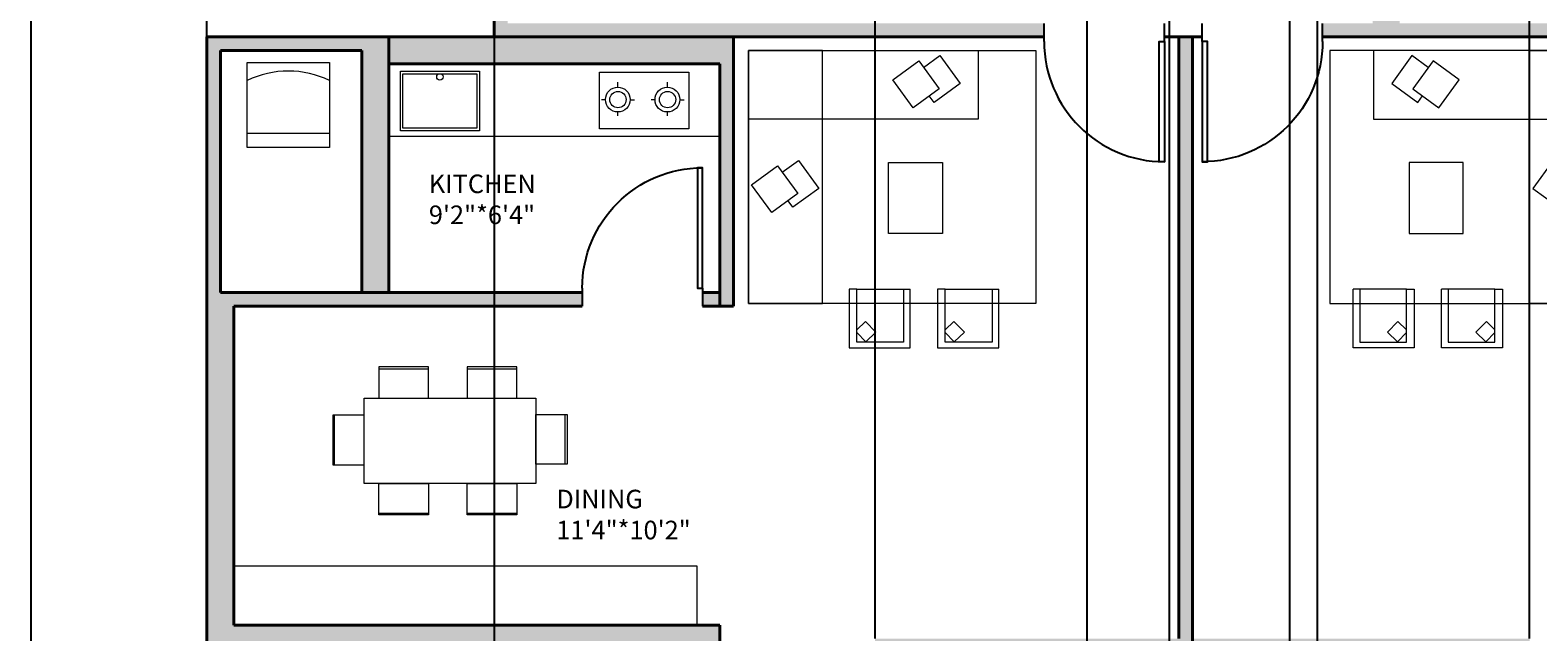
# Model space of a CAD drawing. Units: inches. Extents: x 1642 to 2399, y 1011 to 2291.
# Tile 2 of 7: x 1642 to 2143, y 1395 to 1595. Entities that reach past the tile are written whole.
import ezdxf

# ---------------------------------------------------------------- set-up
doc = ezdxf.new("R2010")
doc.units = ezdxf.units.IN
for name, color, linetype, lineweight in [('A-ANNO-DIMS', 2, 'Continuous', 18), ('A-AREA-IDEN', 7, 'Continuous', 20), ('A-DOOR', 4, 'Continuous', 25), ('A-EQPM', 8, 'Continuous', 18), ('A-FLOR-CASE', 30, 'Continuous', 18), ('A-FLOR-FIXT', 9, 'Continuous', 18), ('A-FURN', 8, 'Continuous', 18), ('A-WALL-PATT', 40, 'Continuous', 13), ('WALL', 40, 'Continuous', 40)]:
    doc.layers.add(name, color=color, linetype=linetype, lineweight=lineweight)
doc.styles.get("Standard").update_dxf_attribs({"font": 'arial.ttf'})
doc.dimstyles.get("Standard").update_dxf_attribs({"dimtxt": 0.18, "dimasz": 0.18, "dimexe": 0.18, "dimexo": 0.0625, "dimgap": 0.09, "dimtad": 0, "dimtih": 1, "dimtoh": 1, "dimdec": 4, "dimzin": 0, "dimdsep": 46, "dimtxsty": 'Standard', "dimcen": 0.09, "dimadec": 0, "dimazin": 0, "dimtfac": 1, "dimtdec": 4, "dimtofl": 0, "dimtmove": 0, "dimatfit": 3, "dimfxl": 1, "dimtolj": 1, "dimtzin": 0, "dimarcsym": 0})

# ---------------------------------------------------------------- blocks, each defined once
blk = doc.blocks.new('*U2')
for p, q in [((0, 0), (0, -6)), ((40, 0), (40, -6))]:
    blk.add_line(p, q)
blk.add_lwpolyline([(0, 0), (0, 40), (1.75, 40), (1.75, 0)], close=True)
blk.add_arc((0, 0), 40, 0, 90)
blk = doc.blocks.new('TABLE-DINING-SIX-SEAT')
for p, q in [((15.31, 48.55), (31.81, 48.55)), ((44.68, 48.55), (61.18, 48.55)), ((0.59, 16.67), (0.59, 33.17)), ((77.22, 16.83), (77.22, 33.33)), ((15.31, 0.59), (31.81, 0.59)), ((44.68, 0.59), (61.18, 0.59))]:
    blk.add_line(p, q)
for points in [[(15.31, 38.77), (31.81, 38.77), (31.81, 49.15), (15.31, 49.15)], [(44.68, 38.77), (61.18, 38.77), (61.18, 49.15), (44.68, 49.15)], [(10.38, 38.77), (67.43, 38.77), (67.43, 10.38), (10.38, 10.38)], [(10.38, 16.67), (10.38, 33.17), (0, 33.17), (0, 16.67)], [(67.43, 16.83), (67.43, 33.33), (77.81, 33.33), (77.81, 16.83)], [(15.31, 10.38), (31.81, 10.38), (31.81, 0), (15.31, 0)], [(44.68, 10.38), (61.18, 10.38), (61.18, 0), (44.68, 0)]]:
    blk.add_lwpolyline(points, close=True)
blk = doc.blocks.new('SEATING-CORNER')
for points in [[(0, 84.13), (76.26, 84.13), (76.26, 61.34), (0, 61.34)], [(0, 0), (24.56, 0), (24.56, 84.13), (0, 84.13)], [(56.51, 80.66), (63.26, 71.39), (54.61, 65.09), (47.86, 74.37)], [(9.57, 45.8), (16.32, 36.53), (7.67, 30.23), (0.92, 39.51)]]:
    blk.add_lwpolyline(points, close=True)
for points in [[(58.1, 78.48), (63.51, 82.42), (70.26, 73.15), (61.61, 66.85), (60.02, 69.03)], [(11.16, 43.62), (16.57, 47.56), (23.32, 38.28), (14.67, 31.99), (13.08, 34.17)]]:
    blk.add_lwpolyline(points)
blk = doc.blocks.new('CHAIR-LOUNGE')
for p, q in [((2.54, 19.51), (0, 19.51)), ((0, 19.51), (0, 0)), ((18.08, 19.51), (20.31, 19.51)), ((20.31, 19.32), (20.31, 19.51)), ((20.31, 0), (20.31, 19.32)), ((0, 0), (20.31, 0))]:
    blk.add_line(p, q)
blk.add_lwpolyline([(2.54, 19.51), (18.08, 19.51), (18.08, 1.93), (2.54, 1.93)], close=True)
blk.add_lwpolyline([(2.54, 6.05), (5.4, 8.82), (8.88, 5.23), (5.55, 2), (2.54, 5.1)])
blk = doc.blocks.new('COOKTOP-TWO-BURNER')
for p, q in [((6.17, 13.89), (6.17, 15.59)), ((22.64, 13.89), (22.64, 15.59)), ((2, 9.67), (0.69, 9.67)), ((6.02, 5.65), (6.02, 4.35)), ((10.24, 9.72), (11.69, 9.72)), ((18.47, 9.67), (17.17, 9.67)), ((22.49, 5.65), (22.49, 4.35)), ((26.71, 9.72), (28.17, 9.72))]:
    blk.add_line(p, q)
blk.add_lwpolyline([(0, 18.89), (29.66, 18.89), (29.66, 0), (0, 0)], close=True)
for centre, radius in [((6.12, 9.77), 4.12), ((6.17, 9.77), 2.71), ((22.59, 9.77), 4.12), ((22.64, 9.77), 2.71)]:
    blk.add_circle(centre, radius)
blk = doc.blocks.new('SINK-KITCHEN-SINGLE')
for points in [[(0, 19.82), (26.24, 19.82), (26.24, 0), (0, 0)], [(0.83, 18.98), (25.41, 18.98), (25.41, 0.83), (0.83, 0.83)]]:
    blk.add_lwpolyline(points, close=True)
blk.add_circle((13.12, 17.93), 1.05)
blk = doc.blocks.new('UTILITY-APPLIANCE')
blk.add_line((0, 4.7), (27.35, 4.7))
blk.add_lwpolyline([(0, 28.26), (27.35, 28.26), (27.35, 0), (0, 0)], close=True)
blk.add_arc((13.68, -6.28), 31.65, 64.3994, 115.6006)
blk = doc.blocks.new('TABLE-COFFEE')
blk.add_lwpolyline([(0, 23.65), (17.89, 23.65), (17.89, 0), (0, 0)], close=True)
blk = doc.blocks.new('*D33')
at = {"layer": 'A-ANNO-DIMS', "color": 0, "lineweight": -2, "transparency": 16777216}
for p, q in [((1700.65, 2232.46), (1642.19, 2232.46)), ((1642.37, 2232.28), (1642.37, 1651.26)), ((1642.37, 1069.89), (1642.37, 1650.9)), ((1700.65, 1069.71), (1642.19, 1069.71))]:
    blk.add_line(p, q, dxfattribs=at)
at = {"layer": 'A-ANNO-DIMS', "color": 0, "transparency": 16777216}
for points in [[(1642.34, 2232.28), (1642.4, 2232.28), (1642.37, 2232.46)], [(1642.34, 1069.89), (1642.4, 1069.89), (1642.37, 1069.71)]]:
    blk.add_solid(points, dxfattribs=at)
at = {"layer": 'Defpoints', "color": 0, "transparency": 16777216}
for p in [(1642.37, 2232.46), (1700.71, 2232.46), (1700.71, 1069.71)]:
    blk.add_point(p, dxfattribs=at)
at = {"layer": 'A-ANNO-DIMS', "color": 0, "transparency": 16777216, "insert": (1642.37, 1651.08), "char_height": 0.18, "attachment_point": 5}
blk.add_mtext('\\A1;1162.7', dxfattribs=at)
blk = doc.blocks.new('*D39')
at = {"layer": 'A-ANNO-DIMS', "color": 0, "lineweight": -2, "transparency": 16777216}
for p, q in [((1700.71, 1592.77), (1700.71, 2290.98)), ((1700.89, 2290.8), (1748.05, 2290.8)), ((1796, 2290.8), (1748.84, 2290.8)), ((1796.18, 1592.77), (1796.18, 2290.98))]:
    blk.add_line(p, q, dxfattribs=at)
at = {"layer": 'A-ANNO-DIMS', "color": 0, "transparency": 16777216}
for points in [[(1700.89, 2290.83), (1700.89, 2290.77), (1700.71, 2290.8)], [(1796, 2290.83), (1796, 2290.77), (1796.18, 2290.8)]]:
    blk.add_solid(points, dxfattribs=at)
at = {"layer": 'Defpoints', "color": 0, "transparency": 16777216}
for p in [(1796.18, 2290.8), (1700.71, 1592.71), (1796.18, 1592.71)]:
    blk.add_point(p, dxfattribs=at)
at = {"layer": 'A-ANNO-DIMS', "color": 0, "transparency": 16777216, "insert": (1748.45, 2290.8), "char_height": 0.18, "attachment_point": 5}
blk.add_mtext('\\A1;95.47', dxfattribs=at)
blk = doc.blocks.new('*D40')
at = {"layer": 'A-ANNO-DIMS', "color": 0, "lineweight": -2, "transparency": 16777216}
for p, q in [((1796.18, 1709.39), (1796.18, 1011.19)), ((2186.88, 1709.39), (2186.88, 1011.19)), ((1796.36, 1011.37), (1991.13, 1011.37)), ((2186.7, 1011.37), (1991.92, 1011.37))]:
    blk.add_line(p, q, dxfattribs=at)
at = {"layer": 'A-ANNO-DIMS', "color": 0, "transparency": 16777216}
for points in [[(1796.36, 1011.4), (1796.36, 1011.34), (1796.18, 1011.37)], [(2186.7, 1011.4), (2186.7, 1011.34), (2186.88, 1011.37)]]:
    blk.add_solid(points, dxfattribs=at)
at = {"layer": 'Defpoints', "color": 0, "transparency": 16777216}
for p in [(1796.18, 1709.46), (2186.88, 1709.46), (2186.88, 1011.37)]:
    blk.add_point(p, dxfattribs=at)
at = {"layer": 'A-ANNO-DIMS', "color": 0, "transparency": 16777216, "insert": (1991.53, 1011.37), "char_height": 0.18, "attachment_point": 5}
blk.add_mtext('\\A1;390.7', dxfattribs=at)
blk = doc.blocks.new('*D46')
at = {"layer": 'A-ANNO-DIMS', "color": 0, "lineweight": -2, "transparency": 16777216}
for p, q in [((2020.45, 1709.39), (2020.45, 1011.19)), ((2060.45, 1709.39), (2060.45, 1011.19)), ((2020.63, 1011.37), (2040.22, 1011.37)), ((2060.27, 1011.37), (2040.67, 1011.37))]:
    blk.add_line(p, q, dxfattribs=at)
at = {"layer": 'A-ANNO-DIMS', "color": 0, "transparency": 16777216}
for points in [[(2020.63, 1011.4), (2020.63, 1011.34), (2020.45, 1011.37)], [(2060.27, 1011.4), (2060.27, 1011.34), (2060.45, 1011.37)]]:
    blk.add_solid(points, dxfattribs=at)
at = {"layer": 'Defpoints', "color": 0, "transparency": 16777216}
for p in [(2020.45, 1709.46), (2060.45, 1709.46), (2060.45, 1011.37)]:
    blk.add_point(p, dxfattribs=at)
at = {"layer": 'A-ANNO-DIMS', "color": 0, "transparency": 16777216, "insert": (2040.45, 1011.37), "char_height": 0.18, "attachment_point": 5}
blk.add_mtext('\\A1;40', dxfattribs=at)
blk = doc.blocks.new('*D48')
at = {"layer": 'A-ANNO-DIMS', "color": 0, "lineweight": -2, "transparency": 16777216}
for p, q in [((1922.74, 1392.77), (1922.74, 2290.98)), ((1922.92, 2290.8), (2031.1, 2290.8)), ((2140.06, 2290.8), (2031.89, 2290.8)), ((2140.24, 1392.77), (2140.24, 2290.98))]:
    blk.add_line(p, q, dxfattribs=at)
at = {"layer": 'A-ANNO-DIMS', "color": 0, "transparency": 16777216}
for points in [[(1922.92, 2290.83), (1922.92, 2290.77), (1922.74, 2290.8)], [(2140.06, 2290.83), (2140.06, 2290.77), (2140.24, 2290.8)]]:
    blk.add_solid(points, dxfattribs=at)
at = {"layer": 'Defpoints', "color": 0, "transparency": 16777216}
for p in [(2140.24, 2290.8), (1922.74, 1392.71), (2140.24, 1392.71)]:
    blk.add_point(p, dxfattribs=at)
at = {"layer": 'A-ANNO-DIMS', "color": 0, "transparency": 16777216, "insert": (2031.49, 2290.8), "char_height": 0.18, "attachment_point": 5}
blk.add_mtext('\\A1;217.5', dxfattribs=at)
blk = doc.blocks.new('*D50')
at = {"layer": 'A-ANNO-DIMS', "color": 0, "lineweight": -2, "transparency": 16777216}
for p, q in [((1993.24, 1295.77), (1993.24, 2290.98)), ((1993.42, 2290.8), (2031.17, 2290.8)), ((2069.56, 2290.8), (2031.82, 2290.8)), ((2069.74, 1295.77), (2069.74, 2290.98))]:
    blk.add_line(p, q, dxfattribs=at)
at = {"layer": 'A-ANNO-DIMS', "color": 0, "transparency": 16777216}
for points in [[(1993.42, 2290.83), (1993.42, 2290.77), (1993.24, 2290.8)], [(2069.56, 2290.83), (2069.56, 2290.77), (2069.74, 2290.8)]]:
    blk.add_solid(points, dxfattribs=at)
at = {"layer": 'Defpoints', "color": 0, "transparency": 16777216}
for p in [(2069.74, 2290.8), (1993.24, 1295.71), (2069.74, 1295.71)]:
    blk.add_point(p, dxfattribs=at)
at = {"layer": 'A-ANNO-DIMS', "color": 0, "transparency": 16777216, "insert": (2031.49, 2290.8), "char_height": 0.18, "attachment_point": 5}
blk.add_mtext('\\A1;76.5', dxfattribs=at)

msp = doc.modelspace()

# ---------------------------------------------------------------- hatches: boundary and pattern name
at = {"layer": 'A-WALL-PATT'}
h = msp.add_hatch(color=256, dxfattribs=at)
h.dxf.hatch_style = 1
h.paths.add_polyline_path([(2340.1804, 2185.4562), (2211.0983, 2185.4562, -0.01876983), (2211.211, 2182.4562), (2211.211, 2176.4562), (2331.211, 2176.4562), (2331.211, 2043.4562), (2171.211, 2043.4562), (2171.211, 2038.9562), (2331.211, 2038.9562), (2331.211, 1916.9562), (2171.211, 1916.9562), (2171.211, 1918.9365), (2166.711, 1918.9365), (2166.711, 1912.4562), (2340.1804, 1912.4562)])
h.paths.add_polyline_path([(2171.211, 2043.4562), (2171.211, 2043.9025), (2170.5217, 2043.9025), (2166.711, 2043.9025), (2166.711, 2038.9562), (2166.711, 1958.9365), (2171.211, 1958.9365)], flags=17)
h.paths.add_polyline_path([(2129.211, 1971.5979), (2124.711, 1971.5979), (2124.711, 1918.4562), (2067.711, 1918.4562), (2067.711, 1913.9562), (2129.211, 1913.9562)])
h.paths.add_polyline_path([(2067.711, 2015.4562), (2124.711, 2015.4562), (2124.711, 2019.9562), (2058.711, 2019.9562), (2058.711, 2015.4562), (2058.711, 1922.9562), (1982.211, 1922.9562), (1982.211, 2015.4562), (1982.211, 2019.9562), (1916.211, 2019.9562), (1916.211, 2070.9562), (1911.711, 2070.9562), (1911.711, 2015.4562), (1911.711, 2012.302), (1916.211, 2012.302), (1916.211, 2015.4562), (1973.211, 2015.4562), (1973.211, 1918.4562), (1973.211, 1913.9562), (2017.1804, 1913.9562), (2067.711, 1913.9562), (2067.711, 1918.4562)])
h.paths.add_polyline_path([(2131.1386, 2075.4562), (2118.1934, 2075.4562), (2118.1934, 2070.9562), (2131.1386, 2070.9562)], flags=17)
h.paths.add_polyline_path([(1918.8034, 2075.4562), (1909.4956, 2075.4562), (1909.4956, 2070.9562), (1918.8034, 2070.9562)], flags=17)
h.paths.add_polyline_path([(1874.211, 2029.9562), (1869.711, 2029.9562), (1869.711, 1960.7404), (1874.211, 1960.7404)], flags=17)
h.paths.add_polyline_path([(1916.211, 1972.302), (1911.711, 1972.302), (1911.711, 1918.4562), (1916.211, 1918.4562)], flags=17)
h.paths.add_polyline_path([(2340.1804, 1912.4562), (2331.1804, 1912.4562), (2331.1804, 1794.4562), (2210.1804, 1794.4562), (2210.1804, 1789.9562), (2279.6804, 1789.9562), (2340.1804, 1789.9562)])
h.paths.add_polyline_path([(2288.6804, 1789.9562), (2279.6804, 1789.9562), (2279.6804, 1785.0846), (2285.6804, 1785.0846), (2288.6804, 1785.0846)], flags=17)
h.paths.add_polyline_path([(2169.6804, 1789.9562), (2170.1804, 1789.9562), (2170.1804, 1794.4562), (2165.1804, 1794.4562), (2165.1804, 1713.9562), (2165.1804, 1709.4562), (2279.6804, 1709.4562), (2279.6804, 1718.4562), (2169.6804, 1718.4562)])
h.paths.add_polyline_path([(2288.6804, 1745.1973, -0.01876983), (2285.6804, 1745.0846), (2279.6804, 1745.0846), (2279.6804, 1709.4562), (2340.1804, 1709.4562), (2340.1804, 1789.9562), (2335.6804, 1789.9562), (2335.6804, 1713.9562), (2288.6804, 1713.9562)])
h.paths.add_polyline_path([(2165.1804, 1713.9562), (2140.6229, 1713.9562), (2088.923, 1713.9562), (2069.7509, 1713.9562), (2060.4457, 1713.9562), (2060.4457, 1709.4562), (2165.1804, 1709.4562)])
h.paths.add_polyline_path([(2020.4457, 1713.9562), (2017.1804, 1713.9562), (2012.6804, 1713.9562), (2009.1946, 1713.9562), (2009.1946, 1709.4562), (2020.4457, 1709.4562)])
h.paths.add_polyline_path([(1969.1946, 1713.9562), (1864.6804, 1713.9562), (1864.6804, 1798.9562), (1860.1804, 1798.9562), (1860.1804, 1792.9562), (1860.1804, 1752.9562), (1860.1804, 1718.4562), (1750.1804, 1718.4562), (1750.1804, 1749.2419), (1744.1804, 1749.2419, -0.01876983), (1741.1804, 1749.3546), (1741.1804, 1709.4562), (1969.1946, 1709.4562)])
h.paths.add_polyline_path([(1741.1804, 1803.4562), (1700.711, 1803.4562), (1700.711, 1794.4562), (1741.1804, 1794.4562)])
h.paths.add_polyline_path([(1820.1804, 1798.9562), (1741.1804, 1798.9562), (1741.1804, 1794.4562), (1741.1804, 1790.0365), (1741.1804, 1789.2419), (1744.1804, 1789.2419), (1750.1804, 1789.2419), (1750.1804, 1794.4562), (1820.1804, 1794.4562)], flags=17)
h.paths.add_polyline_path([(1800.6804, 1709.4562), (1796.1804, 1709.4562), (1796.1804, 1592.7078), (1978.9325, 1592.7078), (1978.9325, 1597.2078), (1800.6804, 1597.2078)])
h.paths.add_polyline_path([(2097.0678, 1709.4562), (2088.0678, 1709.4562), (2088.0678, 1599.6874), (2088.0678, 1597.2078), (2097.0678, 1597.2078)], flags=17)
h.paths.add_polyline_path([(2186.8766, 1709.4562), (2182.3766, 1709.4562), (2182.3766, 1597.2078), (2071.4624, 1597.2078), (2071.4624, 1592.7078), (2186.8766, 1592.7078)])
h.paths.add_polyline_path([(2078.1934, 2075.4562), (2022.711, 2075.4562), (2022.711, 2223.4562), (2166.711, 2223.4562), (2166.711, 2075.4562), (2166.711, 2070.9562), (2171.211, 2070.9562), (2171.211, 2138.8919), (2171.211, 2227.9562), (2335.711, 2227.9562), (2335.711, 2185.4562), (2340.1804, 2185.4562), (2340.1804, 2232.4562), (1874.211, 2232.4562), (1874.211, 2223.4562), (2018.211, 2223.4562), (2018.211, 2075.4562), (1958.8034, 2075.4562), (1958.8034, 2070.9562), (2018.211, 2070.9562), (2018.211, 2019.9562), (1982.211, 2019.9562), (1982.211, 2015.4562), (1982.211, 2010.9562), (2058.711, 2010.9562), (2058.711, 2015.4562), (2058.711, 2019.9562), (2022.711, 2019.9562), (2022.711, 2070.9562), (2078.1934, 2070.9562)])
h.paths.add_polyline_path([(1874.211, 2171.9562), (1874.211, 2176.4562), (1861.9371, 2176.4562), (1861.9371, 2173.4562), (1861.9371, 2167.4562), (1869.711, 2167.4562), (1869.711, 2069.7602), (1874.211, 2069.7602)], flags=17)
h.paths.add_polyline_path([(1705.211, 2227.9562), (1865.211, 2227.9562), (1865.211, 2176.4562), (1874.211, 2176.4562), (1874.211, 2232.4562), (1700.711, 2232.4562), (1700.711, 2176.4562), (1705.211, 2176.4562)])
h.paths.add_polyline_path([(1709.711, 2167.4562), (1821.9371, 2167.4562), (1821.9371, 2173.4562, -0.01876983), (1822.0498, 2176.4562), (1700.711, 2176.4562), (1700.711, 1913.9562), (1860.1804, 1913.9562), (1864.6804, 1913.9562), (1973.211, 1913.9562), (1973.211, 1918.4562), (1916.211, 1918.4562), (1874.211, 1918.4562), (1874.211, 1920.7404), (1869.711, 1920.7404), (1869.711, 1918.4562), (1860.1804, 1918.4562), (1709.711, 1918.4562), (1709.711, 2029.9562), (1874.211, 2029.9562), (1874.211, 2037.0364), (1869.711, 2037.0364), (1869.711, 2034.4562), (1709.711, 2034.4562)])
h.paths.add_polyline_path([(2017.1804, 1913.9562), (2012.6804, 1913.9562), (2012.6804, 1713.9562), (2017.1804, 1713.9562)])
h.paths.add_polyline_path([(1952.4341, 2110.3716), (2000.4134, 2110.3716), (2000.4134, 2133.4189), (1952.4341, 2133.4189)], flags=25)
h.paths.add_polyline_path([(2042.3983, 2110.7121), (2090.3775, 2110.7121), (2090.3775, 2133.7594), (2042.3983, 2133.7594)], flags=25)
h.paths.add_polyline_path([(2201.7332, 2091.8715), (2249.7125, 2091.8715), (2249.7125, 2114.9188), (2201.7332, 2114.9188)], flags=25)
h.paths.add_polyline_path([(1805.186, 2077.6915), (1853.1653, 2077.6915), (1853.1653, 2100.7388), (1805.186, 2100.7388)], flags=25)
h.paths.add_polyline_path([(1794.8897, 1974.6584), (1842.869, 1974.6584), (1842.869, 1997.7057), (1794.8897, 1997.7057)], flags=25)
h.paths.add_polyline_path([(2229.1796, 2204.4209), (2315.1362, 2204.4209), (2315.1362, 2217.1488), (2229.1796, 2217.1488)], flags=25)
h.paths.add_polyline_path([(1715.2159, 2199.5328), (1801.1724, 2199.5328), (1801.1724, 2212.2607), (1715.2159, 2212.2607)], flags=25)
h.paths.add_polyline_path([(2230.7681, 1755.7109), (2271.7283, 1755.7109), (2271.7283, 1778.7582), (2230.7681, 1778.7582)], flags=25)
h.paths.add_polyline_path([(1763.4713, 1764.1742), (1804.4315, 1764.1742), (1804.4315, 1787.2215), (1763.4713, 1787.2215)], flags=25)
h.paths.add_polyline_path([(2076.2643, 1955.0495), (2111.326, 1955.0495), (2111.326, 1978.0968), (2076.2643, 1978.0968)], flags=25)
h.paths.add_polyline_path([(1932.854, 1956.1217), (1967.9158, 1956.1217), (1967.9158, 1979.169), (1932.854, 1979.169)], flags=25)
h.paths.add_polyline_path([(2048.1203, 2031.6107), (2083.1821, 2031.6107), (2083.1821, 2054.658), (2048.1203, 2054.658)], flags=25)
h.paths.add_polyline_path([(2163.5754, 1863.7569), (2208.2347, 1863.7569), (2208.2347, 1886.8042), (2163.5754, 1886.8042)], flags=9)
h.paths.add_polyline_path([(2039.9286, 1809.0957), (2084.5879, 1809.0957), (2084.5879, 1832.143), (2039.9286, 1832.143)], flags=9)
h.paths.add_polyline_path([(1901.0045, 1814.0452), (1945.6638, 1814.0452), (1945.6638, 1837.0925), (1901.0045, 1837.0925)], flags=9)
h.paths.add_polyline_path([(1833.7282, 1852.5627), (1878.3875, 1852.5627), (1878.3875, 1875.61), (1833.7282, 1875.61)], flags=9)
h.paths.add_polyline_path([(2219.1375, 1926.2139), (2267.1167, 1926.2139), (2267.1167, 1949.2612), (2219.1375, 1949.2612)], flags=25)
h.paths.add_polyline_path([(1956.9598, 2029.7735), (1992.0216, 2029.7735), (1992.0216, 2052.8208), (1956.9598, 2052.8208)], flags=25)
h.paths.add_polyline_path([(2229.3, 1523.3399), (2270.2602, 1523.3399), (2270.2602, 1546.3872), (2229.3, 1546.3872)], flags=9)
h.paths.add_polyline_path([(1772.3039, 1526.9922), (1813.2641, 1526.9922), (1813.2641, 1550.0394), (1772.3039, 1550.0394)], flags=9)
h.paths.add_polyline_path([(2172.587, 1420.6999), (2217.2463, 1420.6999), (2217.2463, 1443.7472), (2172.587, 1443.7472)], flags=9)
h.paths.add_polyline_path([(1814.3549, 1422.215), (1859.0143, 1422.215), (1859.0143, 1445.2623), (1814.3549, 1445.2623)], flags=9)
h.paths.add_polyline_path([(2186.0372, 1305.6227), (2234.0165, 1305.6227), (2234.0165, 1328.67), (2186.0372, 1328.67)], flags=9)
h.paths.add_polyline_path([(1756.747, 1349.0694), (1804.7263, 1349.0694), (1804.7263, 1372.1167), (1756.747, 1372.1167)], flags=9)
h.paths.add_polyline_path([(2239.449, 1214.6184), (2287.4282, 1214.6184), (2287.4282, 1237.6657), (2239.449, 1237.6657)], flags=9)
h.paths.add_polyline_path([(1767.104, 1213.8348), (1815.0832, 1213.8348), (1815.0832, 1236.8821), (1767.104, 1236.8821)], flags=9)
h.paths.add_polyline_path([(2046.6809, 1183.6854), (2094.6602, 1183.6854), (2094.6602, 1206.7327), (2046.6809, 1206.7327)], flags=9)
h.paths.add_polyline_path([(1947.2155, 1183.6854), (1995.1948, 1183.6854), (1995.1948, 1206.7327), (1947.2155, 1206.7327)], flags=9)
h.paths.add_polyline_path([(1959.3556, 1258.7871), (1994.4174, 1258.7871), (1994.4174, 1281.8344), (1959.3556, 1281.8344)], flags=9)
h.paths.add_polyline_path([(2049.6419, 1248.9629), (2084.7036, 1248.9629), (2084.7036, 1272.0102), (2049.6419, 1272.0102)], flags=9)
h.paths.add_polyline_path([(2092.7532, 1327.4852), (2127.815, 1327.4852), (2127.815, 1350.5325), (2092.7532, 1350.5325)], flags=9)
h.paths.add_polyline_path([(1944.9358, 1327.4852), (1979.9976, 1327.4852), (1979.9976, 1350.5325), (1944.9358, 1350.5325)], flags=9)
h.paths.add_polyline_path([(1974.5055, 1650.063), (2006.3695, 1650.063), (2006.3695, 1662.7909), (1974.5055, 1662.7909)], flags=9)
h = msp.add_hatch(color=256, dxfattribs=at)
h.dxf.hatch_style = 1
h.paths.add_polyline_path([(2078.7415, 1388.2078), (2028.211, 1388.2078), (2028.211, 1383.7078), (2069.7415, 1383.7078), (2069.7415, 1291.2078), (2069.7415, 1286.7078), (2135.7415, 1286.7078), (2135.7415, 1291.2078), (2078.7415, 1291.2078)])
h.paths.add_polyline_path([(1993.2415, 1383.7078), (2023.711, 1383.7078), (2023.711, 1388.2078), (1984.2415, 1388.2078), (1984.2415, 1291.2078), (1927.2415, 1291.2078), (1927.2415, 1296.6705), (1922.7415, 1296.6705), (1922.7415, 1291.2078), (1922.7415, 1235.7078), (1927.2415, 1235.7078), (1927.2415, 1237.2428), (1927.2415, 1277.2428), (1927.2415, 1286.7078), (1993.2415, 1286.7078), (1993.2415, 1291.2078)])
h.paths.add_polyline_path([(1927.2415, 1388.2078), (1922.7415, 1388.2078), (1922.7415, 1336.6705), (1927.2415, 1336.6705)])
h.paths.add_polyline_path([(1984.2415, 1392.7078), (1922.7415, 1392.7078), (1922.7415, 1388.2078), (1984.2415, 1388.2078)])
h.paths.add_polyline_path([(2023.711, 1392.7078), (1984.2415, 1392.7078), (1984.2415, 1388.2078), (2023.711, 1388.2078)])
h.paths.add_polyline_path([(2078.7415, 1392.7078), (2028.211, 1392.7078), (2028.211, 1388.2078), (2078.7415, 1388.2078)])
h.paths.add_polyline_path([(2140.2415, 1392.7078), (2078.7415, 1392.7078), (2078.7415, 1388.2078), (2135.7415, 1388.2078), (2140.2415, 1388.2078)])
h.paths.add_polyline_path([(2028.211, 1592.7078), (2023.711, 1592.7078), (2023.711, 1392.7078), (2028.211, 1392.7078)])
h.paths.add_polyline_path([(2028.211, 1388.2078), (2023.711, 1388.2078), (2023.711, 1383.7078), (2028.211, 1383.7078)])
h.paths.add_polyline_path([(2028.211, 1392.7078), (2023.711, 1392.7078), (2023.711, 1388.2078), (2028.211, 1388.2078)])
h.paths.add_polyline_path([(2140.2415, 1388.2078), (2135.7415, 1388.2078), (2135.7415, 1332.9578), (2140.2415, 1332.9578)])
h.paths.add_polyline_path([(2069.7415, 1291.2078), (2069.7415, 1295.7078), (2028.211, 1295.7078), (2023.711, 1295.7078), (1993.2415, 1295.7078), (1993.2415, 1291.2078), (1993.2415, 1286.7078), (2029.2415, 1286.7078), (2047.9002, 1286.7078), (2053.9738, 1286.7078), (2069.7415, 1286.7078)])
h.paths.add_polyline_path([(2140.2415, 1291.2078), (2140.2415, 1292.9578), (2135.7415, 1292.9578), (2135.7415, 1269.1323), (2135.7415, 1235.7078), (2140.2415, 1235.7078)])
h.paths.add_polyline_path([(2232.0378, 1392.7078), (2164.6804, 1392.7078), (2164.6804, 1388.2078), (2232.0378, 1388.2078)])
h.paths.add_polyline_path([(2331.1804, 1392.7078), (2232.0378, 1392.7078), (2232.0378, 1388.2078), (2331.1804, 1388.2078)])
h.paths.add_polyline_path([(2340.1804, 1392.7078), (2331.1804, 1392.7078), (2331.1804, 1388.2078), (2340.1804, 1388.2078)])
h.paths.add_polyline_path([(2340.1804, 1388.2078), (2331.1804, 1388.2078), (2331.1804, 1381.9887), (2331.1804, 1266.2078), (2340.1804, 1266.2078)])
h.paths.add_polyline_path([(2331.1804, 1266.2078), (2169.1804, 1266.2078), (2169.1804, 1342.6266), (2164.6804, 1342.6266), (2164.6804, 1266.2078), (2164.6804, 1261.6393), (2168.4442, 1261.6393), (2169.1804, 1261.6393), (2169.1804, 1261.7078), (2331.1804, 1261.7078)])
h.paths.add_polyline_path([(2340.1804, 1266.2078), (2331.1804, 1266.2078), (2331.1804, 1261.7078), (2340.1804, 1261.7078)])
h.paths.add_polyline_path([(2340.1804, 1503.2078), (2331.1804, 1503.2078), (2331.1804, 1392.7078), (2340.1804, 1392.7078)])
h.paths.add_polyline_path([(2340.1804, 1261.7078), (2331.1804, 1261.7078), (2331.1804, 1139.2078), (2331.0462, 1128.7078), (2340.1804, 1128.7078)])
h.paths.add_polyline_path([(2169.1804, 1236.5578, -0.00733557), (2168.4442, 1236.547), (2164.6804, 1236.547), (2164.6804, 1128.7078), (2169.1804, 1128.7078)])
h.paths.add_polyline_path([(2095.1813, 1235.7078), (2028.211, 1235.7078), (2028.211, 1231.2428), (2095.1813, 1231.2428)])
h.paths.add_polyline_path([(2028.211, 1286.7078), (2023.711, 1286.7078), (2023.711, 1235.7078), (2028.211, 1235.7078)])
h.paths.add_polyline_path([(2028.211, 1235.7078), (2023.711, 1235.7078), (2023.711, 1231.2428), (2028.211, 1231.2428)])
h.paths.add_polyline_path([(2023.711, 1235.7078), (1967.2415, 1235.7078), (1967.2415, 1231.2428), (2023.711, 1231.2428)])
h.paths.add_polyline_path([(2028.211, 1231.2428), (2023.711, 1231.2428), (2023.711, 1078.7078), (2028.211, 1078.7078)])
h.paths.add_polyline_path([(1866.711, 1074.2078), (1705.211, 1074.2078), (1705.211, 1119.7078), (1700.711, 1119.7078), (1700.711, 1069.7078), (1866.711, 1069.7078)])
h.paths.add_polyline_path([(2023.711, 1078.7078), (1875.711, 1078.7078), (1875.711, 1074.2078), (1875.711, 1069.7078), (2023.711, 1069.7078)])
h.paths.add_polyline_path([(2028.211, 1078.7078), (2023.711, 1078.7078), (2023.711, 1069.7078), (2028.211, 1069.7078)])
h.paths.add_polyline_path([(2164.6804, 1078.7078), (2028.211, 1078.7078), (2028.211, 1069.7078), (2164.6804, 1069.7078), (2164.6804, 1074.2078)])
h = msp.add_hatch(color=256, dxfattribs=at)
h.dxf.hatch_style = 1
h.paths.add_polyline_path([(1875.711, 1343.4643), (1871.211, 1343.4643), (1871.211, 1266.2078), (1709.711, 1266.2078), (1709.711, 1388.2078), (1700.711, 1388.2078), (1700.711, 1261.7078), (1709.711, 1261.7078), (1875.711, 1261.7078)])
h.paths.add_polyline_path([(1761.211, 1583.7078), (1761.211, 1588.2078), (1761.211, 1592.7078), (1700.711, 1592.7078), (1700.711, 1388.2078), (1709.711, 1388.2078), (1808.8535, 1388.2078), (1871.211, 1388.2078), (1871.211, 1397.2078), (1709.711, 1397.2078), (1709.711, 1503.2078), (1761.211, 1503.2078), (1825.4443, 1503.2078), (1825.4443, 1507.7078), (1761.211, 1507.7078), (1705.211, 1507.7078), (1705.211, 1516.7078), (1705.211, 1588.2078), (1752.211, 1588.2078), (1752.211, 1516.7078), (1752.211, 1507.7078), (1761.211, 1507.7078)])
h.paths.add_polyline_path([(1875.711, 1592.7078), (1761.211, 1592.7078), (1761.211, 1588.2078), (1761.211, 1583.7078), (1871.211, 1583.7078), (1871.211, 1507.7078), (1871.211, 1503.2078), (1875.711, 1503.2078), (1875.711, 1551.7879), (1875.711, 1583.7078)])
h.paths.add_polyline_path([(1823.9074, 1128.7078), (1709.711, 1128.7078), (1709.711, 1261.7078), (1700.711, 1261.7078), (1700.711, 1119.7078), (1705.211, 1119.7078), (1709.711, 1119.7078), (1824.02, 1119.7078, -0.01876983), (1823.9074, 1122.7078)])
h.paths.add_polyline_path([(1875.711, 1236.6154), (1871.9471, 1236.6154, -0.00733557), (1871.211, 1236.6262), (1871.211, 1128.7078), (1863.9074, 1128.7078), (1863.9074, 1122.7078), (1863.9074, 1119.7078), (1866.711, 1119.7078), (1866.711, 1074.2078), (1866.711, 1069.7078), (1875.711, 1069.7078), (1875.711, 1074.2078), (1875.711, 1128.7078)])
h.paths.add_polyline_path([(2173.6804, 1119.7078), (2176.9153, 1119.7078), (2176.9153, 1122.7078), (2176.9153, 1128.7078), (2164.6804, 1128.7078), (2164.6804, 1074.2078), (2164.6804, 1069.7078), (2340.1804, 1069.7078), (2340.1804, 1074.2078), (2335.6804, 1074.2078), (2180.1804, 1074.2078), (2173.6804, 1074.2078)])
h.paths.add_polyline_path([(2340.1804, 1128.7078), (2216.9153, 1128.7078), (2216.9153, 1122.7078, -0.01876983), (2216.8027, 1119.7078), (2340.1804, 1119.7078)], flags=17)
h.paths.add_polyline_path([(2340.1804, 1119.7078), (2335.6804, 1119.7078), (2335.6804, 1074.2078), (2340.1804, 1074.2078)], flags=17)
h.paths.add_polyline_path([(2169.1804, 1592.7078), (2164.6804, 1592.7078), (2164.6804, 1507.7078), (2169.1804, 1507.7078)])
h.paths.add_polyline_path([(2340.1804, 1592.7078), (2169.1804, 1592.7078), (2169.1804, 1588.2078), (2340.1804, 1588.2078)])
h.paths.add_polyline_path([(2340.1804, 1507.7078), (2212.6763, 1507.7078), (2212.6763, 1503.2078), (2340.1804, 1503.2078)])
h.paths.add_polyline_path([(2290.8982, 1588.2078), (2286.3982, 1588.2078), (2286.3982, 1549.1888), (2290.8982, 1549.1888)])
h = msp.add_hatch(color=256, dxfattribs=at)
h.dxf.hatch_style = 1
h.paths.add_polyline_path([(1871.211, 1507.7078), (1865.4443, 1507.7078), (1865.4443, 1503.2078), (1871.211, 1503.2078)])
h.paths.add_polyline_path([(2172.6763, 1507.7078), (2164.6804, 1507.7078), (2164.6804, 1504.0795), (2164.6804, 1503.2078), (2172.6763, 1503.2078)])
h.paths.add_polyline_path([(2290.8982, 1509.1888), (2286.3982, 1509.1888), (2286.3982, 1507.7078), (2290.8982, 1507.7078)])
h.paths.add_polyline_path([(2169.1804, 1388.2078), (2164.6804, 1388.2078), (2164.6804, 1382.6266), (2169.1804, 1382.6266)])
h.paths.add_polyline_path([(2142.989, 1235.7078), (2135.7415, 1235.7078), (2135.1813, 1235.7078), (2135.1813, 1231.2428), (2143.0228, 1231.2428, -0.01396842), (2142.989, 1232.4541)])
h.paths.add_polyline_path([(1927.2415, 1235.7078), (1919.2515, 1235.7078), (1919.2515, 1231.2428), (1926.6813, 1231.2428), (1927.2415, 1231.2428)])
h.paths.add_polyline_path([(1879.2515, 1235.7078), (1875.711, 1235.7078), (1875.711, 1231.2428), (1879.2515, 1231.2428)])

# ---------------------------------------------------------------- linework, layer by layer
at = {"layer": 'A-FLOR-CASE'}
for p, q in [((1761.211, 1583.7078), (1761.211, 1559.7078)), ((1761.211, 1559.7078), (1871.211, 1559.7078)), ((1709.711, 1416.937), (1863.4805, 1416.937)), ((1863.4805, 1416.937), (1863.4805, 1397.2078))]:
    msp.add_line(p, q, dxfattribs=at)
at = {"layer": 'A-FURN'}
for points in [[(1880.749, 1588.2078), (1976.1785, 1588.2078), (1976.1785, 1504.0795), (1880.749, 1504.0795)], [(2164.6804, 1588.2078), (2073.8807, 1588.2078), (2073.8807, 1504.0795), (2164.6804, 1504.0795)]]:
    msp.add_lwpolyline(points, close=True, dxfattribs=at)
at = {"layer": 'WALL'}
for p, q in [((1796.1804, 1709.4562), (1796.1804, 1592.7078)), ((1700.711, 1592.7078), (1747.711, 1592.7078)), ((1700.711, 1592.7078), (1705.211, 1592.7078)), ((1705.211, 1588.2078), (1705.211, 1516.7078)), ((1705.211, 1588.2078), (1752.211, 1588.2078)), ((1752.211, 1588.2078), (1752.211, 1516.7078)), ((1761.211, 1588.2078), (1761.211, 1592.7078)), ((1761.211, 1592.7078), (1761.211, 1583.7078)), ((1761.211, 1588.2078), (1761.211, 1512.2078)), ((1796.1804, 1592.7078), (1978.9325, 1592.7078)), ((1875.711, 1583.7078), (1875.711, 1592.7078)), ((1875.711, 1592.7078), (1978.9325, 1592.7078)), ((2018.9325, 1592.7078), (2023.711, 1592.7078)), ((2018.9325, 1592.7078), (2031.4624, 1592.7078)), ((2023.711, 1592.7078), (2023.711, 1392.7078)), ((2023.711, 1592.7078), (2023.711, 1392.7078)), ((2028.211, 1592.7078), (2028.211, 1388.2078)), ((2028.211, 1592.7078), (2028.211, 1392.7078)), ((2071.4624, 1592.7078), (2186.8766, 1592.7078)), ((1761.211, 1583.7078), (1871.211, 1583.7078)), ((1761.211, 1583.7078), (1761.211, 1507.7078)), ((1871.211, 1583.7078), (1871.211, 1507.7078)), ((1875.711, 1583.7078), (1875.711, 1503.2078)), ((1871.211, 1503.2078), (1871.211, 1551.7879)), ((1875.711, 1503.2078), (1875.711, 1551.7879)), ((1705.211, 1516.7078), (1705.211, 1507.7078)), ((1752.211, 1516.7078), (1752.211, 1507.7078)), ((1761.211, 1507.7078), (1705.211, 1507.7078)), ((1761.211, 1503.2078), (1709.711, 1503.2078)), ((1709.711, 1503.2078), (1709.711, 1397.2078)), ((1761.211, 1507.7078), (1825.4443, 1507.7078)), ((1761.211, 1503.2078), (1825.4443, 1503.2078)), ((1865.4443, 1507.7078), (1871.211, 1507.7078)), ((1865.4443, 1503.2078), (1875.711, 1503.2078)), ((1871.211, 1397.2078), (1709.711, 1397.2078)), ((1871.211, 1388.2078), (1871.211, 1397.2078))]:
    msp.add_line(p, q, dxfattribs=at)
for points in [[(2071.4624, 1592.7078), (2340.1804, 1592.7078), (2340.1804, 1069.7078), (1700.711, 1069.7078), (1700.711, 1592.7078), (1978.9325, 1592.7078)], [(2018.9325, 1592.7078), (2031.4624, 1592.7078)]]:
    msp.add_lwpolyline(points, dxfattribs=at)

# ---------------------------------------------------------------- block references
at = {"layer": 'A-DOOR', "rotation": 180}
msp.add_blockref('*U2', (2018.9325, 1591.2078), dxfattribs=at)
at = {"layer": 'A-DOOR', "xscale": -1, "rotation": 180}
msp.add_blockref('*U2', (2031.4624, 1591.2078), dxfattribs=at)
at = {"layer": 'A-DOOR', "xscale": -1}
msp.add_blockref('*U2', (1865.4443, 1509.2078), dxfattribs=at)
at = {"layer": 'A-EQPM'}
for name, p in [('UTILITY-APPLIANCE', (1714.1264, 1555.9832)), ('COOKTOP-TWO-BURNER', (1831.157, 1562.1069))]:
    msp.add_blockref(name, p, dxfattribs=at)
at = {"layer": 'A-FLOR-FIXT'}
msp.add_blockref('SINK-KITCHEN-SINGLE', (1765.0257, 1561.5046), dxfattribs=at)
at = {"layer": 'A-FURN'}
for name, p in [('SEATING-CORNER', (1880.749, 1504.0795)), ('TABLE-COFFEE', (1927.2558, 1527.3524)), ('CHAIR-LOUNGE', (1914.1494, 1489.331)), ('CHAIR-LOUNGE', (1943.5381, 1489.331)), ('TABLE-DINING-SIX-SEAT', (1742.5854, 1433.8458))]:
    msp.add_blockref(name, p, dxfattribs=at)
at = {"layer": 'A-FURN', "extrusion": (0, 0, -1), "zscale": -1}
for name, p in [('SEATING-CORNER', (-2164.6804, 1504.0795)), ('TABLE-COFFEE', (-2118.1736, 1527.3524)), ('CHAIR-LOUNGE', (-2101.8913, 1489.331)), ('CHAIR-LOUNGE', (-2131.28, 1489.331))]:
    msp.add_blockref(name, p, dxfattribs=at)

# ---------------------------------------------------------------- texts
at = {"layer": 'A-AREA-IDEN', "attachment_point": 1}
for s, insert, char_height in [('KITCHEN\\P9\'2"*6\'4"', (1774.48, 1546.966), 6.17647), ('DINING\\P11\'4"*10\'2"', (1816.8386, 1442.1888), 6.176468)]:
    msp.add_mtext_dynamic_manual_height_columns(s, width=136.850471, gutter_width=30.8823, heights=[0], dxfattribs=dict(at, insert=insert, char_height=char_height))

# ---------------------------------------------------------------- dimensions: what is measured, and where the dimension line sits
at = {"layer": 'A-ANNO-DIMS'}
for base, p1, p2, override, picture, middle in [((1796.1804, 2290.7962), (1700.711, 1592.7078), (1796.1804, 1592.7078), {"dimdec": 2, "dimlfac": 1, "dimrnd": 0, "dimzin": 0, "dimdsep": 46, "dimlunit": 2}, '*D39', (1748.4457, 2290.7962)), ((2140.2415, 2290.7962), (1922.7415, 1392.7078), (2140.2415, 1392.7078), {"dimdec": 1, "dimlfac": 1, "dimrnd": 0, "dimzin": 0, "dimdsep": 46, "dimlunit": 2}, '*D48', (2031.4915, 2290.7962)), ((2069.7415, 2290.7962), (1993.2415, 1295.7078), (2069.7415, 1295.7078), {"dimdec": 1, "dimlfac": 1, "dimrnd": 0, "dimzin": 0, "dimdsep": 46, "dimlunit": 2}, '*D50', (2031.4915, 2290.7962)), ((2186.8766, 1011.3678), (1796.1804, 1709.4562), (2186.8766, 1709.4562), {"dimdec": 1, "dimlfac": 1, "dimrnd": 0, "dimzin": 0, "dimdsep": 46, "dimlunit": 2}, '*D40', (1991.5285, 1011.3678)), ((2060.4457, 1011.3678), (2020.4457, 1709.4562), (2060.4457, 1709.4562), {"dimdec": 0, "dimlfac": 1, "dimrnd": 0, "dimzin": 0, "dimdsep": 46, "dimlunit": 2}, '*D46', (2040.4457, 1011.3678))]:
    dim = msp.add_linear_dim(base=base, p1=p1, p2=p2, dimstyle='Standard', override=override, dxfattribs=at)
    dim.commit()
    dim.dimension.update_dxf_attribs({"geometry": picture, "text_midpoint": middle})
dim = msp.add_linear_dim(base=(1642.371, 2232.4562), p1=(1700.711, 1069.7078), p2=(1700.711, 2232.4562), angle=90, dimstyle='Standard', override={"dimdec": 1, "dimlfac": 1, "dimrnd": 0, "dimzin": 0, "dimdsep": 46, "dimlunit": 2}, dxfattribs=at)
dim.commit()
dim.dimension.update_dxf_attribs({"geometry": '*D33', "text_midpoint": (1642.371, 1651.082)})

doc.saveas('drawing.dxf')
